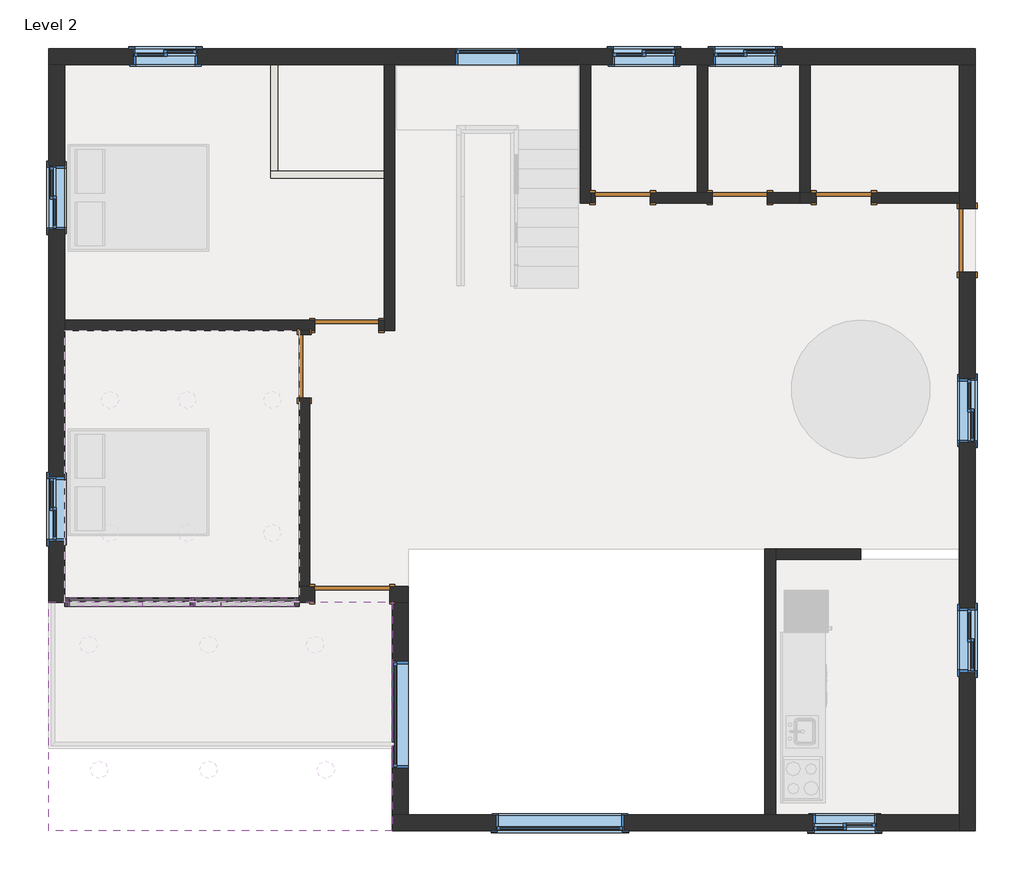
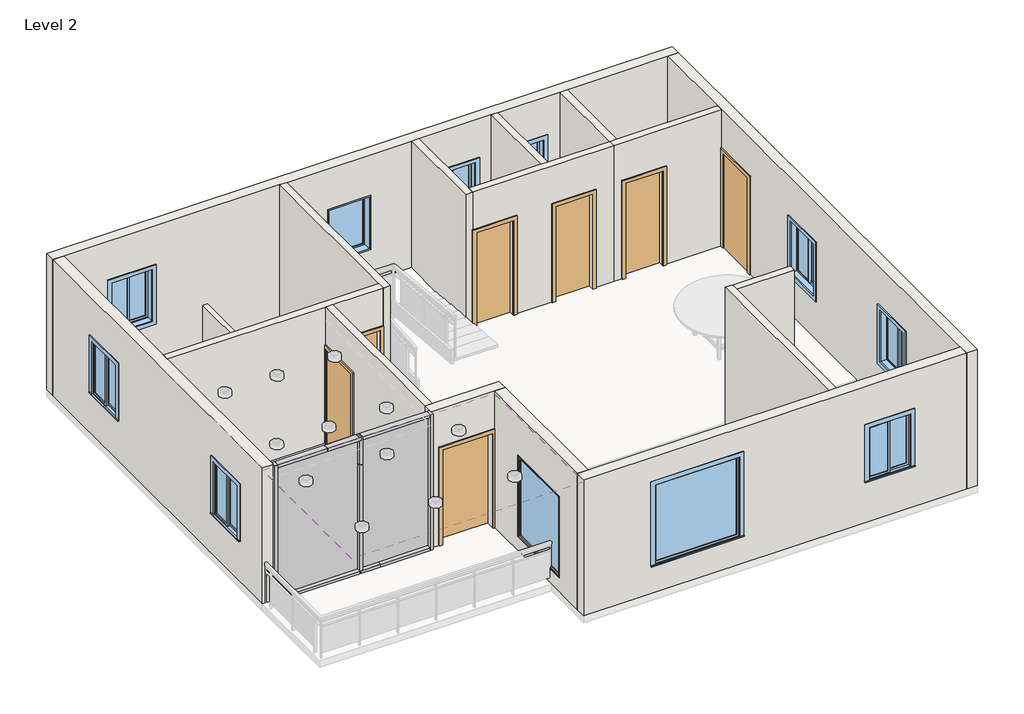
# One storey, part 1 of 2: 18 walls, 11 windows, 10 members, 7 doors, 2 plates, 1 covering.
"""IFC4 building model written with IfcOpenShell, lengths in millimetres."""

from ifc_helpers import new_model, si_unit, frame, origin, place, context, project, spatial, polyline, outline, extrude, faceted_brep, transform, mapped, element, save
from components import door_dc34e247, single_flush_3_5_0848dd25, door_16372e1c, door_0ca8825f, member_89bfb2f9, member_ae70dd35, member_7cfea1b5, member_26d67f61, member_64ee9188, member_eaba9652, member_3f395ae9, system_panel_glazed_5e65faa0, system_panel_glazed_70f543ca, window_4294005a, window_c1f32544, fixed_5_6e519979, window_e25db5b6

model = new_model("IFC4")

# Units and contexts
model_context = context("Model", 3, world=origin())
ifc_project = project(units=[si_unit("LENGTHUNIT", "METRE", prefix="MILLI")], contexts=[model_context])

# Site, building, storey
site = spatial("IfcSite", under=ifc_project)
building = spatial("IfcBuilding", under=site)
storey = spatial("IfcBuildingStorey", under=building, Name="Level 2", Elevation=3200.4)

# Covering
placement = place(None, origin())
element("IfcCovering", 1, ObjectType="2' x 4' ACT System", at=placement, inside=storey, context=model_context, shape_type="SweptSolid", body=[
    extrude(outline(polyline([(-7512.0867944, 6540.7230289), (-7512.0867944, 3264.1230289), (-12426.9867944, 3264.1230289), (-12426.9867944, 6540.7230289), (-7512.0867944, 6540.7230289)])), frame((0.0, 0.0, 6197.6), z_axis=(0.0, 0.0, 1.0), x_axis=(1.0, 0.0, 0.0)), (0.0, 0.0, 1.0), 57.15),
])

# Doors
door_shape = door_dc34e247(model_context)
element("IfcDoor", 2, ObjectType="Single-Flush : 2'7\"", at=placement, inside=storey, context=model_context, shape_type="MappedRepresentation", body=[
    mapped(door_shape, transform((-4212.7737939, 12331.9230289, 3200.4), x_axis=(-1.0, 0.0, 0.0), y_axis=(0.0, -1.0, 0.0), z_axis=(0.0, 0.0, 1.0))),
])
element("IfcDoor", 3, ObjectType="Single-Flush : 2'7\"", at=placement, inside=storey, context=model_context, shape_type="MappedRepresentation", body=[
    mapped(door_shape, transform((-2536.3737939, 12331.9230289, 3200.4), x_axis=(-1.0, 0.0, 0.0), y_axis=(0.0, -1.0, 0.0), z_axis=(0.0, 0.0, 1.0))),
])
element("IfcDoor", 4, ObjectType="Single-Flush : 2'7\"", at=placement, inside=storey, context=model_context, shape_type="MappedRepresentation", body=[
    mapped(door_shape, transform((-1047.7867944, 12331.9230289, 3200.4), x_axis=(-1.0, 0.0, 0.0), y_axis=(0.0, -1.0, 0.0), z_axis=(0.0, 0.0, 1.0))),
])
single_flush_3_5_shape = single_flush_3_5_0848dd25(model_context)
element("IfcDoor", 5, ObjectType="Single-Flush : 3.5'", at=placement, inside=storey, context=model_context, shape_type="MappedRepresentation", body=[
    mapped(single_flush_3_5_shape, transform((-8083.5867944, 6655.0230289, 3200.4), x_axis=(-1.0, 0.0, 0.0), y_axis=(0.0, -1.0, 0.0), z_axis=(0.0, 0.0, 1.0))),
])
door_2_shape = door_16372e1c(model_context)
element("IfcDoor", 6, ObjectType="Single-Flush : 36\" x 84\"", at=placement, inside=storey, context=model_context, shape_type="MappedRepresentation", body=[
    mapped(door_2_shape, transform((-8159.7867944, 10503.1230289, 3200.4), x_axis=(1.0, 0.0, 0.0), y_axis=(0.0, 1.0, 0.0), z_axis=(0.0, 0.0, 1.0))),
])
element("IfcDoor", 7, ObjectType="Single-Flush : 36\" x 84\"", at=placement, inside=storey, context=model_context, shape_type="MappedRepresentation", body=[
    mapped(door_2_shape, transform((-8769.3867944, 9918.9230289, 3200.4), x_axis=(0.0, 1.0, 0.0), y_axis=(-1.0, 0.0, 0.0), z_axis=(0.0, 0.0, 1.0))),
])
door_3_shape = door_0ca8825f(model_context)
element("IfcDoor", 8, ObjectType="Single-Flush : 36\" x 84\"", at=placement, inside=storey, context=model_context, shape_type="MappedRepresentation", body=[
    mapped(door_3_shape, transform((717.5132056, 11722.3230289, 3200.4), x_axis=(0.0, 1.0, 0.0), y_axis=(-1.0, 0.0, 0.0), z_axis=(0.0, 0.0, 1.0))),
])

# Members
member_shape = member_89bfb2f9(model_context)
element("IfcMember", 9, ObjectType="Rectangular Mullion : 2.5\" x 5\" rectangular", at=placement, inside=storey, context=model_context, shape_type="MappedRepresentation", body=[
    mapped(member_shape, transform((-10369.5867944, 6540.7230289, 3263.9), x_axis=(1.0, 0.0, 0.0), y_axis=(0.0, -1.0, 0.0), z_axis=(0.0, 0.0, -1.0))),
])
member_2_shape = member_ae70dd35(model_context)
element("IfcMember", 10, ObjectType="Rectangular Mullion : 2.5\" x 5\" rectangular", at=placement, inside=storey, context=model_context, shape_type="MappedRepresentation", body=[
    mapped(member_2_shape, transform((-10369.5867944, 6540.7230289, 6248.4), x_axis=(0.0, 0.0, 1.0), y_axis=(0.0, -1.0, 0.0), z_axis=(1.0, 0.0, 0.0))),
])
member_3_shape = member_7cfea1b5(model_context)
element("IfcMember", 11, ObjectType="Rectangular Mullion : 2.5\" x 5\" rectangular", at=placement, inside=storey, context=model_context, shape_type="MappedRepresentation", body=[
    mapped(member_3_shape, transform((-10369.5867944, 6540.7230289, 3200.4), x_axis=(0.0, 0.0, -1.0), y_axis=(0.0, -1.0, 0.0), z_axis=(-1.0, 0.0, 0.0))),
])
member_4_shape = member_26d67f61(model_context)
element("IfcMember", 12, ObjectType="Rectangular Mullion : 2.5\" x 5\" rectangular", at=placement, inside=storey, context=model_context, shape_type="MappedRepresentation", body=[
    mapped(member_4_shape, transform((-8909.0867944, 6540.7230289, 6248.4), x_axis=(0.0, 0.0, 1.0), y_axis=(0.0, -1.0, 0.0), z_axis=(1.0, 0.0, 0.0))),
])
member_5_shape = member_64ee9188(model_context)
element("IfcMember", 13, ObjectType="Rectangular Mullion : 2.5\" x 5\" rectangular", at=placement, inside=storey, context=model_context, shape_type="MappedRepresentation", body=[
    mapped(member_5_shape, transform((-10401.3367944, 6540.7230289, 6248.4), x_axis=(0.0, 0.0, 1.0), y_axis=(0.0, -1.0, 0.0), z_axis=(1.0, 0.0, 0.0))),
])
element("IfcMember", 14, ObjectType="Rectangular Mullion : 2.5\" x 5\" rectangular", at=placement, inside=storey, context=model_context, shape_type="MappedRepresentation", body=[
    mapped(member_5_shape, transform((-12134.8867944, 6540.7230289, 3200.4), x_axis=(0.0, 0.0, -1.0), y_axis=(0.0, -1.0, 0.0), z_axis=(-1.0, 0.0, 0.0))),
])
element("IfcMember", 15, ObjectType="Rectangular Mullion : 2.5\" x 5\" rectangular", at=placement, inside=storey, context=model_context, shape_type="MappedRepresentation", body=[
    mapped(member_4_shape, transform((-10337.8367944, 6540.7230289, 3200.4), x_axis=(0.0, 0.0, -1.0), y_axis=(0.0, -1.0, 0.0), z_axis=(-1.0, 0.0, 0.0))),
])
member_6_shape = member_eaba9652(model_context)
element("IfcMember", 16, ObjectType="Rectangular Mullion : 2.5\" x 5\" rectangular", at=placement, inside=storey, context=model_context, shape_type="MappedRepresentation", body=[
    mapped(member_6_shape, transform((-10369.5867944, 6540.7230289, 3200.4), x_axis=(1.0, 0.0, 0.0), y_axis=(0.0, -1.0, 0.0), z_axis=(0.0, 0.0, -1.0))),
])
member_7_shape = member_3f395ae9(model_context)
element("IfcMember", 17, ObjectType="Rectangular Mullion : 2.5\" x 5\" rectangular", at=placement, inside=storey, context=model_context, shape_type="MappedRepresentation", body=[
    mapped(member_7_shape, transform((-8845.5867944, 6540.7230289, 3200.4), x_axis=(1.0, 0.0, 0.0), y_axis=(0.0, -1.0, 0.0), z_axis=(0.0, 0.0, -1.0))),
])
element("IfcMember", 18, ObjectType="Rectangular Mullion : 2.5\" x 5\" rectangular", at=placement, inside=storey, context=model_context, shape_type="MappedRepresentation", body=[
    mapped(member_7_shape, transform((-12198.3867944, 6540.7230289, 6248.4), x_axis=(-1.0, 0.0, 0.0), y_axis=(0.0, -1.0, 0.0), z_axis=(0.0, 0.0, 1.0))),
])

# Plates
system_panel_glazed_shape = system_panel_glazed_5e65faa0(model_context)
element("IfcPlate", 19, ObjectType="System Panel : Glazed", at=placement, inside=storey, context=model_context, shape_type="MappedRepresentation", body=[
    mapped(system_panel_glazed_shape, transform((-11268.1117944, 6540.7230289, 3263.9), x_axis=(1.0, 0.0, 0.0), y_axis=(0.0, 1.0, 0.0), z_axis=(0.0, 0.0, 1.0))),
])
system_panel_glazed_2_shape = system_panel_glazed_70f543ca(model_context)
element("IfcPlate", 20, ObjectType="System Panel : Glazed", at=placement, inside=storey, context=model_context, shape_type="MappedRepresentation", body=[
    mapped(system_panel_glazed_2_shape, transform((-9623.4617944, 6540.7230289, 3263.9), x_axis=(1.0, 0.0, 0.0), y_axis=(0.0, 1.0, 0.0), z_axis=(0.0, 0.0, 1.0))),
])

# Walls
element("IfcWall", 21, ObjectType="4\"", at=placement, inside=storey, context=model_context, shape_type="Brep", body=[
    faceted_brep([(-7626.3867944, 12712.9230289, 3200.4), (-9150.3867944, 12712.9230289, 3200.4), (-9251.9867944, 12712.9230289, 3200.4), (-9251.9867944, 12712.9230289, 4114.8), (-9150.3867944, 12712.9230289, 4114.8), (-7626.3867944, 12712.9230289, 4114.8), (-7626.3867944, 12611.3230289, 3200.4), (-7626.3867944, 12611.3230289, 4114.8), (-9251.9867944, 12611.3230289, 4114.8), (-9251.9867944, 12611.3230289, 3200.4)], [[[0, 1, 2, 3, 4, 5]], [[6, 7, 8, 9]], [[2, 1, 0, 6, 9]], [[5, 4, 3, 8, 7]], [[0, 5, 7, 6]], [[3, 2, 9, 8]]]),
])
element("IfcWall", 22, ObjectType="4\"", at=placement, inside=storey, context=model_context, shape_type="SweptSolid", body=[
    extrude(outline(polyline([(-9150.3867944, 14236.9230289), (-9150.3867944, 12712.9230289), (-9251.9867944, 12712.9230289), (-9251.9867944, 14236.9230289), (-9150.3867944, 14236.9230289)])), frame((0.0, 0.0, 3200.4), z_axis=(0.0, 0.0, 1.0), x_axis=(1.0, 0.0, 0.0)), (0.0, 0.0, 1.0), 914.4),
])
element("IfcWall", 23, ObjectType="6\"", at=placement, inside=storey, context=model_context, shape_type="Brep", body=[
    faceted_brep([(-7626.3867944, 14236.9230289, 3200.4), (-7626.3867944, 12712.9230289, 3200.4), (-7626.3867944, 12611.3230289, 3200.4), (-7626.3867944, 10579.3230289, 3200.4), (-7626.3867944, 10426.9230289, 3200.4), (-7626.3867944, 10426.9230289, 6248.4), (-7626.3867944, 10579.3230289, 6248.4), (-7626.3867944, 14236.9230289, 6248.4), (-7473.9867944, 14236.9230289, 3200.4), (-7473.9867944, 14236.9230289, 6248.4), (-7473.9867944, 10426.9230289, 6248.4), (-7473.9867944, 10426.9230289, 3200.4)], [[[0, 1, 2, 3, 4, 5, 6, 7]], [[8, 9, 10, 11]], [[4, 3, 2, 1, 0, 8, 11]], [[7, 6, 5, 10, 9]], [[0, 7, 9, 8]], [[5, 4, 11, 10]]]),
])
element("IfcWall", 24, ObjectType="6\"", at=placement, inside=storey, context=model_context, shape_type="Brep", body=[
    faceted_brep([(-7626.3867944, 10579.3230289, 3200.4), (-7702.5867944, 10579.3230289, 3200.4), (-7702.5867944, 10579.3230289, 5334.0), (-8616.9867944, 10579.3230289, 5334.0), (-8616.9867944, 10579.3230289, 3200.4), (-12198.3867944, 10579.3230289, 3200.4), (-12198.3867944, 10579.3230289, 6248.4), (-7626.3867944, 10579.3230289, 6248.4), (-7702.5867944, 10426.9230289, 5334.0), (-7702.5867944, 10426.9230289, 3200.4), (-7626.3867944, 10426.9230289, 3200.4), (-7626.3867944, 10426.9230289, 6248.4), (-8693.1867944, 10426.9230289, 6248.4), (-8845.5867944, 10426.9230289, 6248.4), (-12198.3867944, 10426.9230289, 6248.4), (-12198.3867944, 10426.9230289, 3200.4), (-8845.5867944, 10426.9230289, 3200.4), (-8693.1867944, 10426.9230289, 3200.4), (-8616.9867944, 10426.9230289, 3200.4), (-8616.9867944, 10426.9230289, 5334.0)], [[[0, 1, 2, 3, 4, 5, 6, 7]], [[8, 9, 10, 11, 12, 13, 14, 15, 16, 17, 18, 19]], [[10, 9, 1, 0]], [[18, 17, 16, 15, 5, 4]], [[7, 6, 14, 13, 12, 11]], [[0, 7, 11, 10]], [[6, 5, 15, 14]], [[2, 1, 9, 8]], [[3, 2, 8, 19]], [[4, 3, 19, 18]]]),
])
element("IfcWall", 25, ObjectType="6\"", at=placement, inside=storey, context=model_context, shape_type="SweptSolid", body=[
    extrude(outline(polyline([(10426.9230289, 3200.4), (10376.1230289, 3200.4), (10376.1230289, 5334.0), (9461.7230289, 5334.0), (9461.7230289, 3200.4), (6769.3230289, 3200.4), (6769.3230289, 6248.4), (10426.9230289, 6248.4), (10426.9230289, 3200.4)])), frame((-8845.5867944, 0.0, 0.0), z_axis=(1.0, 0.0, 0.0), x_axis=(0.0, 1.0, 0.0)), (0.0, 0.0, 1.0), 152.4),
])
element("IfcWall", 26, ObjectType="6\"", at=placement, inside=storey, context=model_context, shape_type="Brep", body=[
    faceted_brep([(-1441.4867944, 12408.1230289, 5334.0), (-1441.4867944, 12408.1230289, 3200.4), (-1530.3867944, 12408.1230289, 3200.4), (-1682.7867944, 12408.1230289, 3200.4), (-1682.7867944, 12408.1230289, 6248.4), (-1530.3867944, 12408.1230289, 6248.4), (603.2132056, 12408.1230289, 6248.4), (603.2132056, 12408.1230289, 3200.4), (-654.0867944, 12408.1230289, 3200.4), (-654.0867944, 12408.1230289, 5334.0), (-1682.7867944, 12255.7230289, 3200.4), (-1441.4867944, 12255.7230289, 3200.4), (-1441.4867944, 12255.7230289, 5334.0), (-654.0867944, 12255.7230289, 5334.0), (-654.0867944, 12255.7230289, 3200.4), (603.2132056, 12255.7230289, 3200.4), (603.2132056, 12255.7230289, 6248.4), (-1682.7867944, 12255.7230289, 6248.4)], [[[0, 1, 2, 3, 4, 5, 6, 7, 8, 9]], [[10, 11, 12, 13, 14, 15, 16, 17]], [[8, 7, 15, 14]], [[3, 2, 1, 11, 10]], [[6, 5, 4, 17, 16]], [[7, 6, 16, 15]], [[4, 3, 10, 17]], [[12, 11, 1, 0]], [[13, 12, 0, 9]], [[14, 13, 9, 8]]]),
])
element("IfcWall", 27, ObjectType="6\"", at=placement, inside=storey, context=model_context, shape_type="SweptSolid", body=[
    extrude(outline(polyline([(-1530.3867944, 14236.9230289), (-1530.3867944, 12408.1230289), (-1682.7867944, 12408.1230289), (-1682.7867944, 14236.9230289), (-1530.3867944, 14236.9230289)])), frame((0.0, 0.0, 3200.4), z_axis=(0.0, 0.0, 1.0), x_axis=(1.0, 0.0, 0.0)), (0.0, 0.0, 1.0), 3048.0),
])
element("IfcWall", 28, ObjectType="6\"", at=placement, inside=storey, context=model_context, shape_type="Brep", body=[
    faceted_brep([(-4822.3737939, 14236.9230289, 3200.4), (-4822.3737939, 12255.7230289, 3200.4), (-4822.3737939, 12255.7230289, 6248.4), (-4822.3737939, 14236.9230289, 6248.4), (-4669.9737939, 14236.9230289, 3200.4), (-4669.9737939, 14236.9230289, 6248.4), (-4669.9737939, 12408.1230289, 6248.4), (-4669.9737939, 12255.7230289, 6248.4), (-4669.9737939, 12255.7230289, 3200.4), (-4669.9737939, 12408.1230289, 3200.4)], [[[0, 1, 2, 3]], [[4, 5, 6, 7, 8, 9]], [[1, 0, 4, 9, 8]], [[3, 2, 7, 6, 5]], [[2, 1, 8, 7]], [[0, 3, 5, 4]]]),
])
element("IfcWall", 29, ObjectType="6\"", at=placement, inside=storey, context=model_context, shape_type="Brep", body=[
    faceted_brep([(-3819.0737939, 12255.7230289, 3200.4), (-2930.0737939, 12255.7230289, 3200.4), (-2930.0737939, 12255.7230289, 5334.0), (-2142.6737939, 12255.7230289, 5334.0), (-2142.6737939, 12255.7230289, 3200.4), (-1682.7867944, 12255.7230289, 3200.4), (-1682.7867944, 12255.7230289, 6248.4), (-4669.9737939, 12255.7230289, 6248.4), (-4669.9737939, 12255.7230289, 3200.4), (-4606.4737939, 12255.7230289, 3200.4), (-4606.4737939, 12255.7230289, 5334.0), (-3819.0737939, 12255.7230289, 5334.0), (-2930.0737939, 12408.1230289, 5334.0), (-2930.0737939, 12408.1230289, 3200.4), (-2993.5737939, 12408.1230289, 3200.4), (-3145.9737939, 12408.1230289, 3200.4), (-3819.0737939, 12408.1230289, 3200.4), (-3819.0737939, 12408.1230289, 5334.0), (-4606.4737939, 12408.1230289, 5334.0), (-4606.4737939, 12408.1230289, 3200.4), (-4669.9737939, 12408.1230289, 3200.4), (-4669.9737939, 12408.1230289, 6248.4), (-3145.9737939, 12408.1230289, 6248.4), (-2993.5737939, 12408.1230289, 6248.4), (-1682.7867944, 12408.1230289, 6248.4), (-1682.7867944, 12408.1230289, 3200.4), (-2142.6737939, 12408.1230289, 3200.4), (-2142.6737939, 12408.1230289, 5334.0)], [[[0, 1, 2, 3, 4, 5, 6, 7, 8, 9, 10, 11]], [[12, 13, 14, 15, 16, 17, 18, 19, 20, 21, 22, 23, 24, 25, 26, 27]], [[20, 19, 9, 8]], [[26, 25, 5, 4]], [[16, 15, 14, 13, 1, 0]], [[7, 6, 24, 23, 22, 21]], [[8, 7, 21, 20]], [[6, 5, 25, 24]], [[10, 9, 19, 18]], [[11, 10, 18, 17]], [[0, 11, 17, 16]], [[2, 1, 13, 12]], [[3, 2, 12, 27]], [[4, 3, 27, 26]]]),
])
element("IfcWall", 30, ObjectType="6\"", at=placement, inside=storey, context=model_context, shape_type="SweptSolid", body=[
    extrude(outline(polyline([(-2993.5737939, 14236.9230289), (-2993.5737939, 12408.1230289), (-3145.9737939, 12408.1230289), (-3145.9737939, 14236.9230289), (-2993.5737939, 14236.9230289)])), frame((0.0, 0.0, 3200.4), z_axis=(0.0, 0.0, 1.0), x_axis=(1.0, 0.0, 0.0)), (0.0, 0.0, 1.0), 3048.0),
])
element("IfcWall", 31, ObjectType="6\"", at=placement, inside=storey, context=model_context, shape_type="Brep", body=[
    faceted_brep([(-2025.6867944, 3492.7230289, 3200.4), (-2025.6867944, 7150.3230289, 3200.4), (-2025.6867944, 7302.7230289, 3200.4), (-2025.6867944, 7302.7230289, 6248.4), (-2025.6867944, 7150.3230289, 6248.4), (-2025.6867944, 3492.7230289, 6248.4), (-2178.0867944, 3492.7230289, 3200.4), (-2178.0867944, 3492.7230289, 6248.4), (-2178.0867944, 7302.7230289, 6248.4), (-2178.0867944, 7302.7230289, 3200.4)], [[[0, 1, 2, 3, 4, 5]], [[6, 7, 8, 9]], [[2, 1, 0, 6, 9]], [[5, 4, 3, 8, 7]], [[0, 5, 7, 6]], [[3, 2, 9, 8]]]),
])
element("IfcWall", 32, ObjectType="6\"", at=placement, inside=storey, context=model_context, shape_type="SweptSolid", body=[
    extrude(outline(polyline([(-806.4867944, 7150.3230289), (-2025.6867944, 7150.3230289), (-2025.6867944, 7302.7230289), (-806.4867944, 7302.7230289), (-806.4867944, 7150.3230289)])), frame((0.0, 0.0, 3200.4), z_axis=(0.0, 0.0, 1.0), x_axis=(1.0, 0.0, 0.0)), (0.0, 0.0, 1.0), 3048.0),
])
element("IfcWall", 33, ObjectType="9\"", at=placement, inside=storey, context=model_context, shape_type="Brep", body=[
    faceted_brep([(-12426.9867944, 14236.9230289, 3200.4), (-12426.9867944, 6540.7230289, 3200.4), (-12426.9867944, 6540.7230289, 6248.4), (-12426.9867944, 14236.9230289, 6248.4), (-12426.9867944, 8331.4230289, 5334.0), (-12426.9867944, 7417.0230289, 5334.0), (-12426.9867944, 7417.0230289, 4114.8), (-12426.9867944, 8331.4230289, 4114.8), (-12426.9867944, 12789.1230289, 5334.0), (-12426.9867944, 11874.7230289, 5334.0), (-12426.9867944, 11874.7230289, 4114.8), (-12426.9867944, 12789.1230289, 4114.8), (-12198.3867944, 14236.9230289, 3200.4), (-12198.3867944, 14236.9230289, 6248.4), (-12198.3867944, 10579.3230289, 6248.4), (-12198.3867944, 10426.9230289, 6248.4), (-12198.3867944, 6540.7230289, 6248.4), (-12198.3867944, 6540.7230289, 3200.4), (-12198.3867944, 10426.9230289, 3200.4), (-12198.3867944, 10579.3230289, 3200.4), (-12198.3867944, 8331.4230289, 5334.0), (-12198.3867944, 8331.4230289, 4114.8), (-12198.3867944, 7417.0230289, 4114.8), (-12198.3867944, 7417.0230289, 5334.0), (-12198.3867944, 12789.1230289, 5334.0), (-12198.3867944, 12789.1230289, 4114.8), (-12198.3867944, 11874.7230289, 4114.8), (-12198.3867944, 11874.7230289, 5334.0)], [[[0, 1, 2, 3], [4, 5, 6, 7], [8, 9, 10, 11]], [[12, 13, 14, 15, 16, 17, 18, 19], [20, 21, 22, 23], [24, 25, 26, 27]], [[1, 0, 12, 19, 18, 17]], [[2, 1, 17, 16]], [[3, 2, 16, 15, 14, 13]], [[21, 20, 4, 7]], [[22, 21, 7, 6]], [[23, 22, 6, 5]], [[20, 23, 5, 4]], [[25, 24, 8, 11]], [[26, 25, 11, 10]], [[27, 26, 10, 9]], [[24, 27, 9, 8]], [[0, 3, 13, 12]]]),
])
element("IfcWall", 34, ObjectType="9\"", at=placement, inside=storey, context=model_context, shape_type="Brep", body=[
    faceted_brep([(603.2132056, 14236.9230289, 3200.4), (603.2132056, 12408.1230289, 3200.4), (603.2132056, 12255.7230289, 3200.4), (603.2132056, 12179.5230289, 3200.4), (603.2132056, 12179.5230289, 5334.0), (603.2132056, 11265.1230289, 5334.0), (603.2132056, 11265.1230289, 3200.4), (603.2132056, 3492.7230289, 3200.4), (603.2132056, 3264.1230289, 3200.4), (603.2132056, 3264.1230289, 6248.4), (603.2132056, 3492.7230289, 6248.4), (603.2132056, 12255.7230289, 6248.4), (603.2132056, 12408.1230289, 6248.4), (603.2132056, 14236.9230289, 6248.4), (603.2132056, 5537.4230289, 5334.0), (603.2132056, 5537.4230289, 4114.8), (603.2132056, 6451.8230289, 4114.8), (603.2132056, 6451.8230289, 5334.0), (603.2132056, 8826.7230289, 5334.0), (603.2132056, 8826.7230289, 4114.8), (603.2132056, 9741.1230289, 4114.8), (603.2132056, 9741.1230289, 5334.0), (831.8132056, 12179.5230289, 5334.0), (831.8132056, 12179.5230289, 3200.4), (831.8132056, 14236.9230289, 3200.4), (831.8132056, 14236.9230289, 6248.4), (831.8132056, 3264.1230289, 6248.4), (831.8132056, 3264.1230289, 3200.4), (831.8132056, 11265.1230289, 3200.4), (831.8132056, 11265.1230289, 5334.0), (831.8132056, 5537.4230289, 5334.0), (831.8132056, 6451.8230289, 5334.0), (831.8132056, 6451.8230289, 4114.8), (831.8132056, 5537.4230289, 4114.8), (831.8132056, 8826.7230289, 5334.0), (831.8132056, 9741.1230289, 5334.0), (831.8132056, 9741.1230289, 4114.8), (831.8132056, 8826.7230289, 4114.8)], [[[0, 1, 2, 3, 4, 5, 6, 7, 8, 9, 10, 11, 12, 13], [14, 15, 16, 17], [18, 19, 20, 21]], [[22, 23, 24, 25, 26, 27, 28, 29], [30, 31, 32, 33], [34, 35, 36, 37]], [[28, 27, 8, 7, 6]], [[24, 23, 3, 2, 1, 0]], [[13, 12, 11, 10, 9, 26, 25]], [[0, 13, 25, 24]], [[9, 8, 27, 26]], [[4, 3, 23, 22]], [[5, 4, 22, 29]], [[6, 5, 29, 28]], [[15, 14, 30, 33]], [[16, 15, 33, 32]], [[17, 16, 32, 31]], [[14, 17, 31, 30]], [[19, 18, 34, 37]], [[20, 19, 37, 36]], [[21, 20, 36, 35]], [[18, 21, 35, 34]]]),
])
element("IfcWall", 35, ObjectType="9\"", at=placement, inside=storey, context=model_context, shape_type="Brep", body=[
    faceted_brep([(603.2132056, 3492.7230289, 3200.4), (-2025.6867944, 3492.7230289, 3200.4), (-2178.0867944, 3492.7230289, 3200.4), (-7283.4867944, 3492.7230289, 3200.4), (-7512.0867944, 3492.7230289, 3200.4), (-7512.0867944, 3492.7230289, 6248.4), (-7283.4867944, 3492.7230289, 6248.4), (-2178.0867944, 3492.7230289, 6248.4), (-2025.6867944, 3492.7230289, 6248.4), (603.2132056, 3492.7230289, 6248.4), (-1492.2867944, 3492.7230289, 5334.0), (-1492.2867944, 3492.7230289, 4114.8), (-577.8867944, 3492.7230289, 4114.8), (-577.8867944, 3492.7230289, 5334.0), (-6026.1867944, 3492.7230289, 5638.8), (-6026.1867944, 3492.7230289, 3810.0), (-4197.3867944, 3492.7230289, 3810.0), (-4197.3867944, 3492.7230289, 5638.8), (603.2132056, 3264.1230289, 3200.4), (603.2132056, 3264.1230289, 6248.4), (-7512.0867944, 3264.1230289, 6248.4), (-7512.0867944, 3264.1230289, 3200.4), (-1492.2867944, 3264.1230289, 5334.0), (-577.8867944, 3264.1230289, 5334.0), (-577.8867944, 3264.1230289, 4114.8), (-1492.2867944, 3264.1230289, 4114.8), (-6026.1867944, 3264.1230289, 5638.8), (-4197.3867944, 3264.1230289, 5638.8), (-4197.3867944, 3264.1230289, 3810.0), (-6026.1867944, 3264.1230289, 3810.0)], [[[0, 1, 2, 3, 4, 5, 6, 7, 8, 9], [10, 11, 12, 13], [14, 15, 16, 17]], [[18, 19, 20, 21], [22, 23, 24, 25], [26, 27, 28, 29]], [[4, 3, 2, 1, 0, 18, 21]], [[9, 8, 7, 6, 5, 20, 19]], [[0, 9, 19, 18]], [[5, 4, 21, 20]], [[11, 10, 22, 25]], [[12, 11, 25, 24]], [[13, 12, 24, 23]], [[10, 13, 23, 22]], [[15, 14, 26, 29]], [[16, 15, 29, 28]], [[17, 16, 28, 27]], [[14, 17, 27, 26]]]),
])
element("IfcWall", 36, ObjectType="9\"", at=placement, inside=storey, context=model_context, shape_type="SweptSolid", body=[
    extrude(outline(polyline([(6540.7230289, 3200.4), (3492.7230289, 3200.4), (3492.7230289, 6248.4), (6540.7230289, 6248.4), (6540.7230289, 3200.4)]), holes=[polyline([(4165.8230289, 3505.2), (5689.8230289, 3505.2), (5689.8230289, 5334.0), (4165.8230289, 5334.0), (4165.8230289, 3505.2)])]), frame((-7512.0867944, 0.0, 0.0), z_axis=(1.0, 0.0, 0.0), x_axis=(0.0, 1.0, 0.0)), (0.0, 0.0, 1.0), 228.6),
])
element("IfcWall", 37, ObjectType="9\"", at=placement, inside=storey, context=model_context, shape_type="Brep", body=[
    faceted_brep([(-12426.9867944, 14236.9230289, 3200.4), (-12198.3867944, 14236.9230289, 3200.4), (-9251.9867944, 14236.9230289, 3200.4), (-9150.3867944, 14236.9230289, 3200.4), (-7626.3867944, 14236.9230289, 3200.4), (-7473.9867944, 14236.9230289, 3200.4), (-4822.3737939, 14236.9230289, 3200.4), (-4669.9737939, 14236.9230289, 3200.4), (-3145.9737939, 14236.9230289, 3200.4), (-2993.5737939, 14236.9230289, 3200.4), (-1682.7867944, 14236.9230289, 3200.4), (-1530.3867944, 14236.9230289, 3200.4), (603.2132056, 14236.9230289, 3200.4), (831.8132056, 14236.9230289, 3200.4), (831.8132056, 14236.9230289, 6248.4), (603.2132056, 14236.9230289, 6248.4), (-1530.3867944, 14236.9230289, 6248.4), (-1682.7867944, 14236.9230289, 6248.4), (-2993.5737939, 14236.9230289, 6248.4), (-3145.9737939, 14236.9230289, 6248.4), (-4669.9737939, 14236.9230289, 6248.4), (-4822.3737939, 14236.9230289, 6248.4), (-7473.9867944, 14236.9230289, 6248.4), (-7626.3867944, 14236.9230289, 6248.4), (-12198.3867944, 14236.9230289, 6248.4), (-12426.9867944, 14236.9230289, 6248.4), (-10299.7367944, 14236.9230289, 5334.0), (-10299.7367944, 14236.9230289, 4114.8), (-11214.1367944, 14236.9230289, 4114.8), (-11214.1367944, 14236.9230289, 5334.0), (-2002.9737939, 14236.9230289, 5334.0), (-2002.9737939, 14236.9230289, 4114.8), (-2917.3737939, 14236.9230289, 4114.8), (-2917.3737939, 14236.9230289, 5334.0), (-3450.7737939, 14236.9230289, 5334.0), (-3450.7737939, 14236.9230289, 4114.8), (-4365.1737939, 14236.9230289, 4114.8), (-4365.1737939, 14236.9230289, 5334.0), (-5690.9802942, 14236.9230289, 5334.0), (-5690.9802942, 14236.9230289, 4114.8), (-6605.3802942, 14236.9230289, 4114.8), (-6605.3802942, 14236.9230289, 5334.0), (-12426.9867944, 14465.5230289, 3200.4), (-12426.9867944, 14465.5230289, 6248.4), (831.8132056, 14465.5230289, 6248.4), (831.8132056, 14465.5230289, 3200.4), (-10299.7367944, 14465.5230289, 5334.0), (-11214.1367944, 14465.5230289, 5334.0), (-11214.1367944, 14465.5230289, 4114.8), (-10299.7367944, 14465.5230289, 4114.8), (-2002.9737939, 14465.5230289, 5334.0), (-2917.3737939, 14465.5230289, 5334.0), (-2917.3737939, 14465.5230289, 4114.8), (-2002.9737939, 14465.5230289, 4114.8), (-3450.7737939, 14465.5230289, 5334.0), (-4365.1737939, 14465.5230289, 5334.0), (-4365.1737939, 14465.5230289, 4114.8), (-3450.7737939, 14465.5230289, 4114.8), (-5690.9802942, 14465.5230289, 5334.0), (-6605.3802942, 14465.5230289, 5334.0), (-6605.3802942, 14465.5230289, 4114.8), (-5690.9802942, 14465.5230289, 4114.8)], [[[0, 1, 2, 3, 4, 5, 6, 7, 8, 9, 10, 11, 12, 13, 14, 15, 16, 17, 18, 19, 20, 21, 22, 23, 24, 25], [26, 27, 28, 29], [30, 31, 32, 33], [34, 35, 36, 37], [38, 39, 40, 41]], [[42, 43, 44, 45], [46, 47, 48, 49], [50, 51, 52, 53], [54, 55, 56, 57], [58, 59, 60, 61]], [[13, 12, 11, 10, 9, 8, 7, 6, 5, 4, 3, 2, 1, 0, 42, 45]], [[14, 13, 45, 44]], [[25, 24, 23, 22, 21, 20, 19, 18, 17, 16, 15, 14, 44, 43]], [[26, 29, 47, 46]], [[29, 28, 48, 47]], [[28, 27, 49, 48]], [[27, 26, 46, 49]], [[30, 33, 51, 50]], [[33, 32, 52, 51]], [[32, 31, 53, 52]], [[31, 30, 50, 53]], [[34, 37, 55, 54]], [[37, 36, 56, 55]], [[36, 35, 57, 56]], [[35, 34, 54, 57]], [[38, 41, 59, 58]], [[41, 40, 60, 59]], [[40, 39, 61, 60]], [[39, 38, 58, 61]], [[0, 25, 43, 42]]]),
])
element("IfcWall", 38, ObjectType="9\"", at=placement, inside=storey, context=model_context, shape_type="Brep", body=[
    faceted_brep([(-8845.5867944, 6540.7230289, 3200.4), (-8616.9867944, 6540.7230289, 3200.4), (-8616.9867944, 6540.7230289, 5334.0), (-7550.1867944, 6540.7230289, 5334.0), (-7550.1867944, 6540.7230289, 3200.4), (-7512.0867944, 6540.7230289, 3200.4), (-7283.4867944, 6540.7230289, 3200.4), (-7283.4867944, 6540.7230289, 6248.4), (-7512.0867944, 6540.7230289, 6248.4), (-8845.5867944, 6540.7230289, 6248.4), (-8616.9867944, 6769.3230289, 5334.0), (-8616.9867944, 6769.3230289, 3200.4), (-8693.1867944, 6769.3230289, 3200.4), (-8845.5867944, 6769.3230289, 3200.4), (-8845.5867944, 6769.3230289, 6248.4), (-8693.1867944, 6769.3230289, 6248.4), (-7283.4867944, 6769.3230289, 6248.4), (-7283.4867944, 6769.3230289, 3200.4), (-7550.1867944, 6769.3230289, 3200.4), (-7550.1867944, 6769.3230289, 5334.0)], [[[0, 1, 2, 3, 4, 5, 6, 7, 8, 9]], [[10, 11, 12, 13, 14, 15, 16, 17, 18, 19]], [[18, 17, 6, 5, 4]], [[13, 12, 11, 1, 0]], [[9, 8, 7, 16, 15, 14]], [[0, 9, 14, 13]], [[7, 6, 17, 16]], [[4, 3, 19, 18]], [[3, 2, 10, 19]], [[2, 1, 11, 10]]]),
])

# Windows
window_shape = window_4294005a(model_context)
element("IfcWindow", 39, ObjectType="Casement with Trim : 72\" x 72\"", at=placement, inside=storey, context=model_context, shape_type="MappedRepresentation", body=[
    mapped(window_shape, transform((-5111.7867944, 3378.4230289, 3200.4), x_axis=(-1.0, 0.0, 0.0), y_axis=(0.0, -1.0, 0.0), z_axis=(0.0, 0.0, 1.0))),
])
window_2_shape = window_c1f32544(model_context)
element("IfcWindow", 40, ObjectType="Fixed : 36\" x 48\"", at=placement, inside=storey, context=model_context, shape_type="MappedRepresentation", body=[
    mapped(window_2_shape, transform((-6110.0802942, 14351.2230289, 3200.4), x_axis=(1.0, 0.0, 0.0), y_axis=(0.0, 1.0, 0.0), z_axis=(0.0, 0.0, 1.0))),
])
fixed_5_shape = fixed_5_6e519979(model_context)
element("IfcWindow", 41, ObjectType="Fixed : 5'", at=placement, inside=storey, context=model_context, shape_type="MappedRepresentation", body=[
    mapped(fixed_5_shape, transform((-7397.7867944, 4889.7230289, 3200.4), x_axis=(0.0, -1.0, 0.0), y_axis=(1.0, 0.0, 0.0), z_axis=(0.0, 0.0, 1.0))),
])
window_3_shape = window_e25db5b6(model_context)
element("IfcWindow", 42, ObjectType="Slider with Trim : 36\" x 48\"", at=placement, inside=storey, context=model_context, shape_type="MappedRepresentation", body=[
    mapped(window_3_shape, transform((-12312.6867944, 7874.2230289, 3200.4), x_axis=(0.0, 1.0, 0.0), y_axis=(-1.0, 0.0, 0.0), z_axis=(0.0, 0.0, 1.0))),
])
element("IfcWindow", 43, ObjectType="Slider with Trim : 36\" x 48\"", at=placement, inside=storey, context=model_context, shape_type="MappedRepresentation", body=[
    mapped(window_3_shape, transform((-12312.6867944, 12331.9230289, 3200.4), x_axis=(0.0, 1.0, 0.0), y_axis=(-1.0, 0.0, 0.0), z_axis=(0.0, 0.0, 1.0))),
])
element("IfcWindow", 44, ObjectType="Slider with Trim : 36\" x 48\"", at=placement, inside=storey, context=model_context, shape_type="MappedRepresentation", body=[
    mapped(window_3_shape, transform((-10756.9367944, 14351.2230289, 3200.4), x_axis=(1.0, 0.0, 0.0), y_axis=(0.0, 1.0, 0.0), z_axis=(0.0, 0.0, 1.0))),
])
element("IfcWindow", 45, ObjectType="Slider with Trim : 36\" x 48\"", at=placement, inside=storey, context=model_context, shape_type="MappedRepresentation", body=[
    mapped(window_3_shape, transform((-1035.0867944, 3378.4230289, 3200.4), x_axis=(-1.0, 0.0, 0.0), y_axis=(0.0, -1.0, 0.0), z_axis=(0.0, 0.0, 1.0))),
])
element("IfcWindow", 46, ObjectType="Slider with Trim : 36\" x 48\"", at=placement, inside=storey, context=model_context, shape_type="MappedRepresentation", body=[
    mapped(window_3_shape, transform((717.5132056, 5994.6230289, 3200.4), x_axis=(0.0, -1.0, 0.0), y_axis=(1.0, 0.0, 0.0), z_axis=(0.0, 0.0, 1.0))),
])
element("IfcWindow", 47, ObjectType="Slider with Trim : 36\" x 48\"", at=placement, inside=storey, context=model_context, shape_type="MappedRepresentation", body=[
    mapped(window_3_shape, transform((717.5132056, 9283.9230289, 3200.4), x_axis=(0.0, -1.0, 0.0), y_axis=(1.0, 0.0, 0.0), z_axis=(0.0, 0.0, 1.0))),
])
element("IfcWindow", 48, ObjectType="Slider with Trim : 36\" x 48\"", at=placement, inside=storey, context=model_context, shape_type="MappedRepresentation", body=[
    mapped(window_3_shape, transform((-2460.1737939, 14351.2230289, 3200.4), x_axis=(1.0, 0.0, 0.0), y_axis=(0.0, 1.0, 0.0), z_axis=(0.0, 0.0, 1.0))),
])
element("IfcWindow", 49, ObjectType="Slider with Trim : 36\" x 48\"", at=placement, inside=storey, context=model_context, shape_type="MappedRepresentation", body=[
    mapped(window_3_shape, transform((-3907.9737939, 14351.2230289, 3200.4), x_axis=(1.0, 0.0, 0.0), y_axis=(0.0, 1.0, 0.0), z_axis=(0.0, 0.0, 1.0))),
])

save(model, "model.ifc")

# Revit data of these elements
# Type "2' x 4' ACT System"
#   Assembly Code = "C3030210"
#   built-in parameter 1002203 = 1 (stored number, unit not read)
#   built-in parameter 1002202 = 1 (stored number, unit not read)
#   Layers, outside or top first: 0' - 1 5/8" "Default" (function 1); 0' - 0 5/8" "Softwood, Lumber" (function 5)
# Type "Single-Flush : 2'7\""
#   Type Mark = "8"
#   Construction Type Id = "MDOOR"
#   Assembly Code = "C1020"
#   Analytic Construction = "Metal"
#   Thickness = 0' - 2"
#   Heat Transfer Coefficient (U) = 0.651978 BTU/(h·ft²·°F)
#   Height = 7' - 0"
#   Trim Projection Ext = 0' - 1"
#   Trim Projection Int = 0' - 1"
#   Trim Width = 0' - 3"
#   Width = 2' - 7"
#   Define Thermal Properties by = 1
#   Door Material = Door - Panel
#   Frame Material = Door - Frame
#   Visual Light Transmittance = 0
#   Solar Heat Gain Coefficient = 0
#   Function = (empty or 0)
#   Wall Closure = (empty or 0)
# Type "Single-Flush : 3.5'"
#   Type Mark = "10"
#   Construction Type Id = "MDOOR"
#   Assembly Code = "C1020"
#   Analytic Construction = "Metal"
#   Thickness = 0' - 2"
#   Heat Transfer Coefficient (U) = 0.651978 BTU/(h·ft²·°F)
#   Height = 7' - 0"
#   Trim Projection Ext = 0' - 1"
#   Trim Projection Int = 0' - 1"
#   Trim Width = 0' - 3"
#   Width = 3' - 6"
#   Define Thermal Properties by = 1
#   Door Material = Door - Panel
#   Frame Material = Door - Frame
#   Visual Light Transmittance = 0
#   Solar Heat Gain Coefficient = 0
#   Function = (empty or 0)
#   Wall Closure = (empty or 0)
# Type "Single-Flush : 36\" x 84\""
#   Type Mark = "1"
#   Construction Type Id = "MDOOR"
#   Assembly Code = "C1020"
#   Analytic Construction = "Metal"
#   Thickness = 0' - 2"
#   Heat Transfer Coefficient (U) = 0.651978 BTU/(h·ft²·°F)
#   Height = 7' - 0"
#   Trim Projection Ext = 0' - 1"
#   Trim Projection Int = 0' - 1"
#   Trim Width = 0' - 3"
#   Width = 3' - 0"
#   Define Thermal Properties by = 1
#   Door Material = Door - Panel
#   Frame Material = Door - Frame
#   Visual Light Transmittance = 0
#   Solar Heat Gain Coefficient = 0
#   Function = (empty or 0)
#   Wall Closure = (empty or 0)
# Type "Rectangular Mullion : 2.5\" x 5\" rectangular"
#   built-in parameter 1007304 = 0.416667 (stored number, unit not read)
#   built-in parameter 1007301 = 0.104167 (stored number, unit not read)
#   built-in parameter 1007300 = 0.104167 (stored number, unit not read)
# Type "System Panel : Glazed"
#   Construction Type Id = "GSP4R"
#   Analytic Construction = "1/8 in Pilkington single glazing"
#   Visual Light Transmittance = 0.9
#   Solar Heat Gain Coefficient = 0.86
#   Heat Transfer Coefficient (U) = 1.18115 BTU/(h·ft²·°F)
# Type "4\""
#   Assembly Code = "B2010"
#   Layers, outside or top first: 0' - 4" "EXT WALL" (function 1)
# Type "6\""
#   Assembly Code = "B2010"
#   Layers, outside or top first: 0' - 6" "INT WALL" (function 1)
# Type "9\""
#   Assembly Code = "B2010"
#   Layers, outside or top first: 0' - 9" "EXT WALL" (function 1)
# Type "Casement with Trim : 72\" x 72\""
#   Type Mark = "18"
#   Construction Type Id = "GSP4R"
#   Assembly Code = "B2020100"
#   Analytic Construction = "1/8 in Pilkington single glazing"
#   Visual Light Transmittance = 0.9
#   Solar Heat Gain Coefficient = 0.78
#   Heat Transfer Coefficient (U) = 0.6496 BTU/(h·ft²·°F)
#   Height = 6' - 0"
#   Default Sill Height = 2' - 0"
#   Trim Projection - Ext. = 0' - 0 1/2"
#   Trim Projection - Int. = 0' - 0 3/4"
#   Trim Width - Exterior = 0' - 3 1/2"
#   Trim Width - Interior = 0' - 3 1/2"
#   Width = 6' - 0"
#   Window Inset = 0' - 0 3/4"
#   Define Thermal Properties by = 1
#   Glass Pane Material = Glass
#   Sash Material = Stainless Steel
#   Trim Exterior Material = Stainless Steel
#   Trim Interior Material = Steel, Polished
#   Wall Closure = (empty or 0)
# Type "Fixed : 36\" x 48\""
#   Type Mark = "9"
#   Construction Type Id = "GSP4R"
#   Assembly Code = "B2020100"
#   Analytic Construction = "1/8 in Pilkington single glazing"
#   Visual Light Transmittance = 0.9
#   Solar Heat Gain Coefficient = 0.78
#   Heat Transfer Coefficient (U) = 0.6496 BTU/(h·ft²·°F)
#   Height = 4' - 0"
#   Default Sill Height = 3' - 0"
#   Width = 3' - 0"
#   Window Inset = 0' - 0 3/4"
#   Define Thermal Properties by = 1
#   Wall Closure = 3
#   Glass Pane Material = Glass
#   Sash Material = Sash
# Type "Fixed : 5'"
#   Type Mark = "16"
#   Construction Type Id = "GSP4R"
#   Assembly Code = "B2020100"
#   Analytic Construction = "1/8 in Pilkington single glazing"
#   Visual Light Transmittance = 0.9
#   Solar Heat Gain Coefficient = 0.78
#   Heat Transfer Coefficient (U) = 0.6496 BTU/(h·ft²·°F)
#   Height = 6' - 0"
#   Default Sill Height = 1' - 0"
#   Width = 5' - 0"
#   Window Inset = 0' - 0 3/4"
#   Define Thermal Properties by = 1
#   Glass Pane Material = Glass
#   Sash Material = Sash
#   Wall Closure = (empty or 0)
# Type "Slider with Trim : 36\" x 48\""
#   Type Mark = "10"
#   Construction Type Id = "GSP4R"
#   Assembly Code = "B2020100"
#   Analytic Construction = "1/8 in Pilkington single glazing"
#   Visual Light Transmittance = 0.9
#   Solar Heat Gain Coefficient = 0.78
#   Heat Transfer Coefficient (U) = 0.6496 BTU/(h·ft²·°F)
#   Height = 4' - 0"
#   Default Sill Height = 3' - 0"
#   Trim Projection - Ext. = 0' - 0 3/4"
#   Trim Projection - Int. = 0' - 0 3/4"
#   Trim Width - Exterior = 0' - 3 1/2"
#   Trim Width - Interior = 0' - 3 1/2"
#   Width = 3' - 0"
#   Window Inset = 0' - 0 3/4"
#   Define Thermal Properties by = 1
#   Glass Pane Material = Glass
#   Sash Material = Sash
#   Trim Exterior Material = Trim
#   Trim Interior Material = Trim
#   Wall Closure = (empty or 0)
# Element 1 (IfcCovering, "2' x 4' ACT System")
#   Height Offset From Level = 9' - 10"
#   Phase Created = New Construction
#   Materials on its faces: "Softwood, Lumber", "Default"
# Elements 2, 3, 4 (IfcDoor, "Single-Flush : 2'7\"")
#   Phase Created = New Construction
#   Materials on its faces: "Door - Frame", "Door - Panel"
# Element 5 (IfcDoor, "Single-Flush : 3.5'")
#   Phase Created = New Construction
#   Materials on its faces: "Door - Frame", "Door - Panel"
# Elements 6, 7, 8 (IfcDoor, "Single-Flush : 36\" x 84\"")
#   Phase Created = New Construction
#   Materials on its faces: "Door - Frame", "Door - Panel"
# Elements 9, 10, 11, 12, 13, 14, 15, 16, 17, 18 (IfcMember, "Rectangular Mullion : 2.5\" x 5\" rectangular")
#   Phase Created = New Construction
#   Materials on its faces: "Aluminum"
# Elements 19, 20 (IfcPlate, "System Panel : Glazed")
#   Phase Created = New Construction
#   Materials on its faces: "Glass"
# Elements 21, 22 (IfcWall, "4\"")
#   Top Offset = 0' - 0"
#   Base Offset = 0' - 0"
#   Unconnected Height = 3' - 0"
#   wall height = 3' - 0"
#   Phase Created = New Construction
#   Base Constraint = Level 2
#   Materials on its faces: "EXT WALL"
# Elements 23, 24, 25, 26, 27, 28, 29, 30, 31, 32 (IfcWall, "6\"")
#   Top Offset = 0' - 0"
#   Base Offset = 0' - 0"
#   Unconnected Height = 10' - 0"
#   wall height = 10' - 0"
#   Phase Created = New Construction
#   Base Constraint = Level 2
#   Materials on its faces: "INT WALL"
# Elements 33, 34, 35, 36, 37, 38 (IfcWall, "9\"")
#   Top Offset = 0' - 0"
#   Base Offset = 0' - 0"
#   Unconnected Height = 10' - 0"
#   wall height = 10' - 0"
#   Phase Created = New Construction
#   Base Constraint = Level 2
#   Materials on its faces: "EXT WALL"
# Element 39 (IfcWindow, "Casement with Trim : 72\" x 72\"")
#   Mark = "27"
#   Phase Created = New Construction
#   Materials on its faces: "Stainless Steel", "Steel, Polished", "Glass"
# Element 40 (IfcWindow, "Fixed : 36\" x 48\"")
#   Mark = "23"
#   Phase Created = New Construction
#   Materials on its faces: "Sash", "Glass"
# Element 41 (IfcWindow, "Fixed : 5'")
#   Mark = "25"
#   Phase Created = New Construction
#   Materials on its faces: "Sash", "Glass"
# Element 42 (IfcWindow, "Slider with Trim : 36\" x 48\"")
#   Mark = "14"
#   Phase Created = New Construction
#   Materials on its faces: "Sash", "Trim", "Glass"
# Element 43 (IfcWindow, "Slider with Trim : 36\" x 48\"")
#   Mark = "15"
#   Phase Created = New Construction
#   Materials on its faces: "Sash", "Trim", "Glass"
# Element 44 (IfcWindow, "Slider with Trim : 36\" x 48\"")
#   Mark = "16"
#   Phase Created = New Construction
#   Materials on its faces: "Sash", "Trim", "Glass"
# Element 45 (IfcWindow, "Slider with Trim : 36\" x 48\"")
#   Mark = "18"
#   Phase Created = New Construction
#   Materials on its faces: "Sash", "Trim", "Glass"
# Element 46 (IfcWindow, "Slider with Trim : 36\" x 48\"")
#   Mark = "19"
#   Phase Created = New Construction
#   Materials on its faces: "Sash", "Trim", "Glass"
# Element 47 (IfcWindow, "Slider with Trim : 36\" x 48\"")
#   Mark = "20"
#   Phase Created = New Construction
#   Materials on its faces: "Sash", "Trim", "Glass"
# Element 48 (IfcWindow, "Slider with Trim : 36\" x 48\"")
#   Mark = "21"
#   Phase Created = New Construction
#   Materials on its faces: "Sash", "Trim", "Glass"
# Element 49 (IfcWindow, "Slider with Trim : 36\" x 48\"")
#   Mark = "22"
#   Phase Created = New Construction
#   Materials on its faces: "Sash", "Trim", "Glass"
# Materials
#   "Default": colour RGB 127 127 127, transparency 0
#   "Softwood, Lumber": class "Wood", colour RGB 144 112 60, transparency 0, Description = "Pinus Echinata", Cost = 0
#   "Door - Panel": class "Wood", colour RGB 210 159 95, transparency 0
#   "Door - Frame": colour RGB 118 70 51, transparency 0
#   "EXT WALL": class "Generic", colour RGB 159 125 47, transparency 0, Cost = 0
#   "INT WALL": class "Generic", colour RGB 187 179 160, transparency 0, Cost = 0
#   "Glass": class "Glass", colour RGB 0 128 192, transparency 0.75, Description = "Soda Lime Glass", Cost = 0
#   "Stainless Steel": class "Metal", colour RGB 0 0 0, transparency 0, Description = "Stainless Steel 18/8", Cost = 0
#   "Steel, Polished": class "Metal", colour RGB 57 57 57, transparency 0, Description = "Polished steel", Cost = 0
#   "Sash": class "Wood", colour RGB 224 178 126, transparency 0
#   "Trim": class "Wood", colour RGB 224 178 126, transparency 0
#   "Aluminum": class "Metal", colour RGB 247 247 247, transparency 0, Description = "Aluminum 6061", Cost = 0
